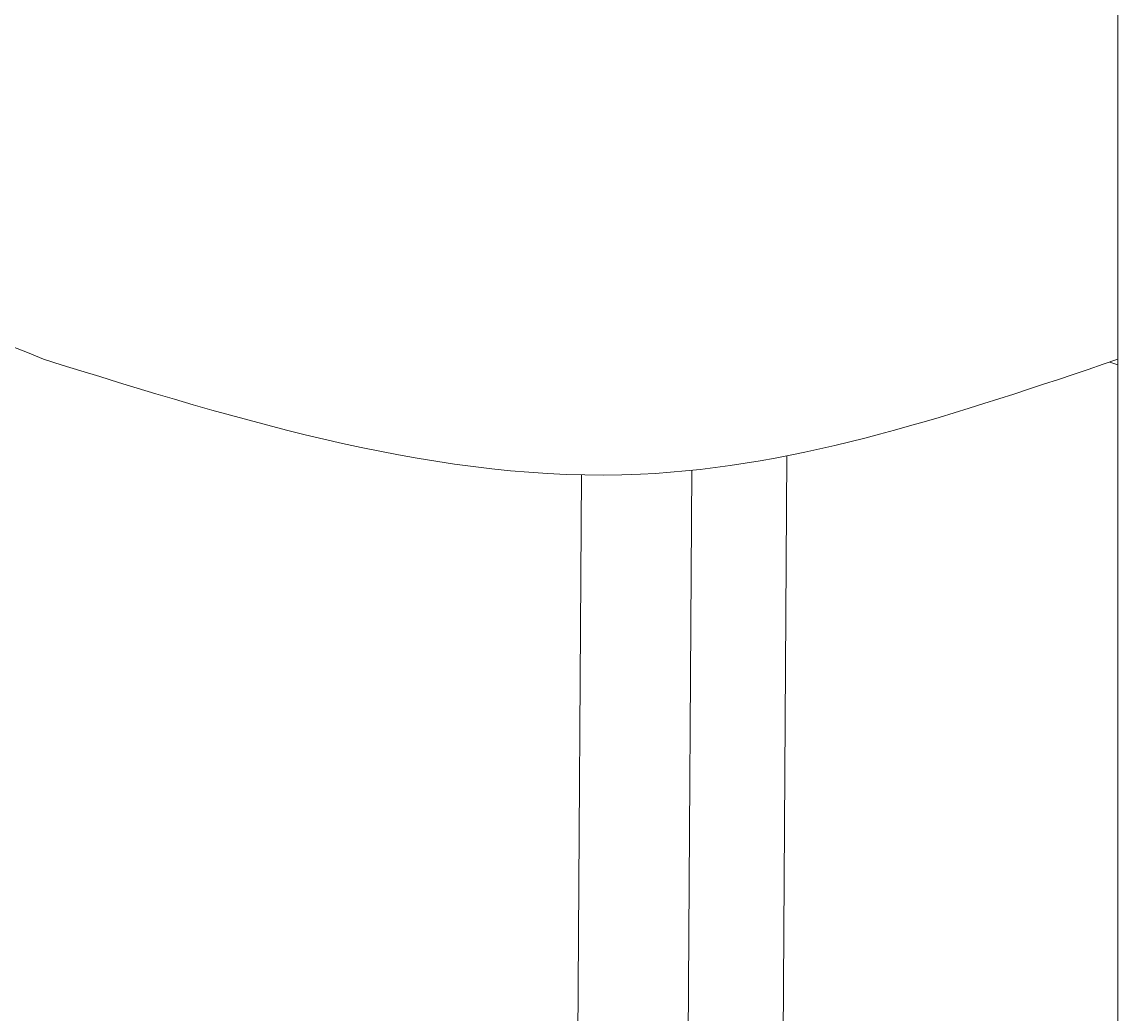
# Model space of a CAD drawing. Units: inches. Extents: x -46 to 1145, y -527 to 760.
# Tile 40 of 57: x 83 to 114, y 597 to 625. Entities that reach past the tile are written whole.
import ezdxf

# ---------------------------------------------------------------- set-up
doc = ezdxf.new("R2010")
doc.units = ezdxf.units.IN
doc.header["$MEASUREMENT"] = 0
doc.layers.add('A-ANNO-DIMS', color=2, linetype='Continuous', lineweight=18)
doc.layers.add('A-FURN', color=2, linetype='Continuous', lineweight=13)
doc.styles.get("Standard").update_dxf_attribs({"font": 'arial.ttf'})
doc.dimstyles.get("Standard").update_dxf_attribs({"dimtxt": 0.18, "dimasz": 0.18, "dimexe": 0.18, "dimexo": 0.0625, "dimgap": 0.09, "dimtad": 0, "dimtih": 1, "dimtoh": 1, "dimdec": 0, "dimzin": 0, "dimdsep": 46, "dimlunit": 3, "dimtxsty": 'Standard', "dimcen": 0.09, "dimadec": 0, "dimazin": 0, "dimtfac": 1, "dimtdec": 0, "dimtofl": 0, "dimtmove": 0, "dimatfit": 3, "dimfxl": 1, "dimtolj": 1, "dimtzin": 0, "dimarcsym": 0})

# ---------------------------------------------------------------- blocks, each defined once
blk = doc.blocks.new('BED-QUEEN-FURNISHED')
for p, q in [((60, 80), (60, 0)), ((50.463, 0), (50.758, 45.907)), ((44.724, 0), (45.016, 45.372)), ((47.804, 0), (48.097, 45.499))]:
    blk.add_line(p, q)
for centre, radius, start, end in [((15, 13.075), 38.562, 67.1089, 112.8911), ((40.884, -5.132), 56.884, 70.3635, 70.606)]:
    blk.add_arc(centre, radius, start, end)
blk.add_open_spline([(30, 48.601), (35.57, 46.869), (45.642, 43.737), (55.565, 47.098), (60, 48.601)], degree=3, knots=[0, 0, 0, 0, 16.971495, 30.687365, 30.687365, 30.687365, 30.687365])
blk = doc.blocks.new('*D652')
at = {"layer": 'A-ANNO-DIMS', "color": 0, "lineweight": -2, "transparency": 16777216}
for p, q in [((113.972, 646.503), (126.09, 646.503)), ((125.91, 646.323), (125.91, 606.691)), ((125.91, 566.683), (125.91, 606.314)), ((113.972, 566.503), (126.09, 566.503))]:
    blk.add_line(p, q, dxfattribs=at)
at = {"layer": 'A-ANNO-DIMS', "color": 0, "transparency": 16777216}
for points in [[(125.88, 646.323), (125.94, 646.323), (125.91, 646.503)], [(125.88, 566.683), (125.94, 566.683), (125.91, 566.503)]]:
    blk.add_solid(points, dxfattribs=at)
at = {"layer": 'Defpoints', "color": 0, "transparency": 16777216}
for p in [(113.91, 646.503), (125.91, 646.503), (113.91, 566.503)]:
    blk.add_point(p, dxfattribs=at)
at = {"layer": 'A-ANNO-DIMS', "color": 0, "transparency": 16777216, "insert": (125.91, 606.503), "char_height": 0.18, "attachment_point": 5}
blk.add_mtext('\\A1;QUEEN BED 80 TYP.', dxfattribs=at)
blk = doc.blocks.new('*D685')
at = {"layer": 'A-ANNO-DIMS', "color": 0, "lineweight": -2, "transparency": 16777216}
for p, q in [((183.501, 700.889), (-46.216, 700.889)), ((-46.036, 700.709), (-46.036, 116.385)), ((-46.036, -468.302), (-46.036, 116.021)), ((12.501, -468.482), (-46.216, -468.482))]:
    blk.add_line(p, q, dxfattribs=at)
at = {"layer": 'A-ANNO-DIMS', "color": 0, "transparency": 16777216}
for points in [[(-46.066, 700.709), (-46.006, 700.709), (-46.036, 700.889)], [(-46.066, -468.302), (-46.006, -468.302), (-46.036, -468.482)]]:
    blk.add_solid(points, dxfattribs=at)
at = {"layer": 'Defpoints', "color": 0, "transparency": 16777216}
for p in [(-46.036, 700.889), (183.564, 700.889), (12.564, -468.482)]:
    blk.add_point(p, dxfattribs=at)
at = {"layer": 'A-ANNO-DIMS', "color": 0, "transparency": 16777216, "insert": (-46.036, 116.203), "char_height": 0.18, "attachment_point": 5}
blk.add_mtext('\\A1;1169.4', dxfattribs=at)

msp = doc.modelspace()

# ---------------------------------------------------------------- block references
at = {"layer": 'A-FURN'}
msp.add_blockref('BED-QUEEN-FURNISHED', (53.91, 566.503), dxfattribs=at)

# ---------------------------------------------------------------- dimensions: what is measured, and where the dimension line sits
at = {"layer": 'A-ANNO-DIMS'}
dim = msp.add_linear_dim(base=(-46.0363, 700.8886), p1=(12.5637, -468.4824), p2=(183.5637, 700.8886), angle=90, dimstyle='Standard', override={"dimdec": 1, "dimlfac": 1, "dimrnd": 0, "dimzin": 0, "dimdsep": 46, "dimlunit": 2}, dxfattribs=at)
dim.commit()
dim.dimension.update_dxf_attribs({"geometry": '*D685', "text_midpoint": (-46.0363, 116.2031)})
dim = msp.add_linear_dim(base=(125.9098, 646.5029), p1=(113.9098, 566.5028), p2=(113.9098, 646.5029), angle=90, text='QUEEN BED <> TYP.', dimstyle='Standard', override={"dimdec": 0, "dimlfac": 1, "dimrnd": 0, "dimzin": 0, "dimdsep": 46, "dimlunit": 2}, dxfattribs=at)
dim.commit()
dim.dimension.update_dxf_attribs({"geometry": '*D652', "text_midpoint": (125.9098, 606.5028)})

doc.saveas('drawing.dxf')
